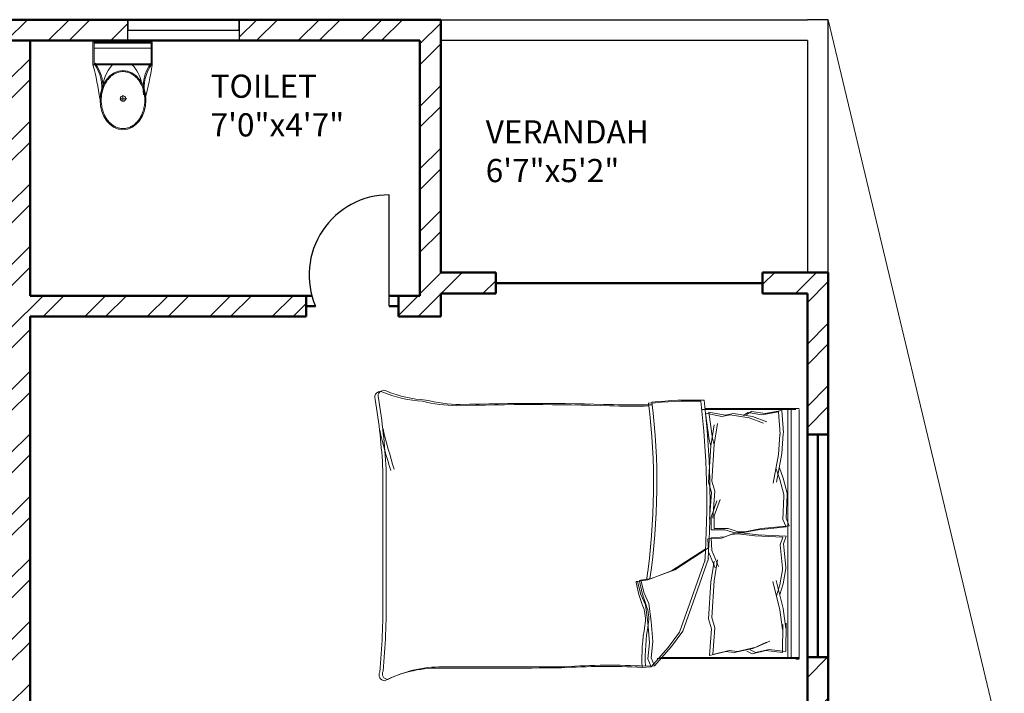
# Model space of a CAD drawing. Units: inches. Extents: x 1901 to 2863, y 888 to 2433.
# Tile 65 of 91: x 2169 to 2381, y 2129 to 2274. Entities that reach past the tile are written whole.
import ezdxf

# ---------------------------------------------------------------- set-up
doc = ezdxf.new("R2010")
doc.units = ezdxf.units.IN
for name, color, linetype, lineweight in [('A-ANNO-SYMB', 8, 'Continuous', 13), ('A-AREA-IDEN', 7, 'Continuous', 18), ('A-DOOR', 4, 'Continuous', 25), ('A-FLOR-FIXT', 9, 'Continuous', 18), ('A-FLOR-HRAL', 41, 'Continuous', 25), ('A-FURN', 8, 'Continuous', 18), ('A-GLAZ', 3, 'Continuous', 25), ('A-WALL', 7, 'Continuous', 50), ('A-WALL-PATT', 8, 'Continuous', 13)]:
    doc.layers.add(name, color=color, linetype=linetype, lineweight=lineweight)
doc.styles.get("Standard").update_dxf_attribs({"font": 'arial.ttf'})

# ---------------------------------------------------------------- blocks, each defined once
blk = doc.blocks.new('A$C31115884')
for p, q in [((257.5, 466.4), (257.5, 523.2)), ((283.1, 497.7), (223.4, 497.7)), ((0, 200), (0, 0)), ((520, 200), (0, 200)), ((10, 190), (10, 10)), ((510, 190), (10, 190)), ((510, 10), (510, 190)), ((520, 0), (520, 200)), ((510, 54.5), (0, 54.5)), ((10, 10), (510, 10)), ((0, 0), (520, 0))]:
    blk.add_line(p, q)
blk.add_circle((255.6, 496.4), 23.6)
for centre, radius, start, end in [((2777.7, -204.6), 2807, 165.4549, 171.71327), ((-294.5, 403.3), 364.7, 324.20913, 9.34987), ((-294.5, 403.3), 374.7, 324.20913, 9.34987), ((805.8, 403.3), 364.7, 170.65013, 215.79087), ((3237, 905), 2807, 188.28673, 194.5451), ((383.6, 406.2), 293.5, 190.27735, 224.15636), ((139.5, 406.2), 293.5, 315.84364, 2.65635), ((805.8, 403.3), 374.7, 179.20365, 215.79087)]:
    blk.add_arc(centre, radius, start, end)
blk.add_ellipse((256.2, 509.9), major_axis=(0, -260.7), ratio=0.772727)
blk.add_open_spline([(256.2, 259.2), (263.1, 259.2), (270, 259.7), (287.8, 262.3), (298.7, 265.1), (319.9, 273.1), (330.2, 278.4), (350.1, 291.1), (359.7, 298.7), (377.7, 315.9), (386.2, 325.5), (401.7, 346.6), (408.8, 358.1), (421.3, 382.5), (426.8, 395.5), (435.9, 422.4), (439.5, 436.4), (444.8, 465.1), (446.5, 479.7), (447.9, 509.2), (447.6, 524), (445, 553.3), (442.7, 567.8), (436.3, 596), (432.1, 609.7), (421.9, 636), (416, 648.6), (402.5, 672.1), (395, 683), (378.6, 703), (369.8, 712.1), (351.1, 728), (341.3, 734.8), (320.9, 746.2), (310.4, 750.7), (288.9, 757.3), (278, 759.4), (256, 761), (245, 760.6), (223.1, 757.2), (212.3, 754.3), (191.1, 746.1), (180.8, 740.7), (160.9, 727.8), (151.4, 720.1), (133.5, 702.7), (125.1, 693), (109.6, 671.7), (102.6, 660.2), (90.2, 635.7), (84.9, 622.7), (76, 595.6), (72.4, 581.6), (67.2, 552.9), (65.6, 538.2), (64.4, 508.8), (64.8, 494), (67.5, 464.7), (69.9, 450.2), (76.6, 422), (80.8, 408.3), (91.1, 382.2), (97.2, 369.7), (110.8, 346.3), (118.4, 335.4), (134.8, 315.6), (143.7, 306.7), (162.4, 290.9), (172.3, 284.2), (192.8, 273), (203.3, 268.6), (224.8, 262.2), (235.8, 260.2), (249.9, 259.3), (253, 259.2), (256.2, 259.2)], degree=3, knots=[0, 0, 0, 0, 0.110105, 0.110105, 0.285049, 0.285049, 0.459994, 0.459994, 0.634938, 0.634938, 0.809882, 0.809882, 0.984827, 0.984827, 1.159771, 1.159771, 1.334715, 1.334715, 1.50966, 1.50966, 1.684604, 1.684604, 1.859549, 1.859549, 2.034493, 2.034493, 2.209437, 2.209437, 2.384382, 2.384382, 2.559326, 2.559326, 2.73427, 2.73427, 2.909215, 2.909215, 3.084159, 3.084159, 3.259103, 3.259103, 3.434048, 3.434048, 3.608992, 3.608992, 3.783936, 3.783936, 3.958881, 3.958881, 4.133825, 4.133825, 4.30877, 4.30877, 4.483714, 4.483714, 4.658658, 4.658658, 4.833603, 4.833603, 5.008547, 5.008547, 5.183491, 5.183491, 5.358436, 5.358436, 5.53338, 5.53338, 5.708324, 5.708324, 5.883269, 5.883269, 6.058213, 6.058213, 6.233158, 6.233158, 6.283185, 6.283185, 6.283185, 6.283185])
blk = doc.blocks.new('BED-DOUBLE')
for p, q in [((31.9, 59.58), (28.25, 55.42)), ((31.9, 59.58), (28.25, 55.42)), ((33.85, 59.67), (31.9, 59.58, 4.35)), ((33.85, 59.67), (31.9, 59.58, 4.35)), ((32.59, 57.85), (31.9, 59.58)), ((32.59, 57.85), (31.9, 59.58)), ((0.03, 57.78), (0.03, 4.12)), ((0.74, 57.78), (30.62, 57.78)), ((0.74, 57.78), (30.62, 57.78)), ((31.18, 59.32), (27.53, 55.16)), ((31.18, 59.32), (27.53, 55.16)), ((33.14, 59.41), (31.18, 59.32, 4.35)), ((33.14, 59.41), (31.18, 59.32, 4.35)), ((31.87, 57.59), (31.18, 59.32)), ((31.87, 57.59), (31.18, 59.32)), ((31.53, 54.12), (31.87, 57.59)), ((31.53, 54.12), (31.87, 57.59)), ((32.24, 54.37), (32.59, 57.85)), ((32.24, 54.37), (32.59, 57.85)), ((2.9, 56.23), (2.79, 50.16)), ((2.9, 56.23), (2.79, 50.16)), ((2.9, 56.23), (6.5, 55.8)), ((2.9, 56.23), (6.5, 55.8)), ((3.61, 56.48), (3.51, 50.42)), ((3.61, 56.48), (3.51, 50.42)), ((3.61, 56.48), (7.22, 56.06)), ((3.61, 56.48), (7.22, 56.06)), ((9.3, 55.33), (6.29, 54)), ((9.3, 55.33), (6.29, 54)), ((6.5, 55.8), (9.39, 56.47)), ((6.5, 55.8), (9.39, 56.47)), ((10.01, 55.58), (7.01, 54.26)), ((10.01, 55.58), (7.01, 54.26)), ((7.22, 56.06), (10.11, 56.73)), ((7.22, 56.06), (10.11, 56.73)), ((13.31, 56.23), (9.3, 55.33)), ((13.31, 56.23), (9.3, 55.33)), ((9.39, 56.47), (10.56, 55.89)), ((9.39, 56.47), (10.56, 55.89)), ((14.02, 56.48), (10.01, 55.58)), ((14.02, 56.48), (10.01, 55.58)), ((10.11, 56.73), (11.28, 56.15)), ((10.11, 56.73), (11.28, 56.15)), ((15.11, 56.01), (13.31, 56.23)), ((15.11, 56.01), (13.31, 56.23)), ((15.83, 56.27), (14.02, 56.48)), ((15.83, 56.27), (14.02, 56.48)), ((18.63, 56.89), (15.11, 56.01)), ((18.63, 56.88), (15.11, 56.01)), ((19.35, 57.14), (15.83, 56.27)), ((19.35, 57.14), (15.83, 56.27)), ((18.18, 51.12), (18.63, 56.89)), ((18.18, 51.12), (18.63, 56.88)), ((18.9, 51.38), (19.35, 57.14)), ((18.9, 51.38), (19.35, 57.14)), ((28.25, 55.42), (25.81, 52.11)), ((28.25, 55.42), (25.81, 52.11)), ((27.53, 55.16), (25.1, 51.86)), ((27.53, 55.16), (25.1, 51.86)), ((31.87, 49.77), (31.53, 54.12)), ((31.87, 49.77), (31.53, 54.12)), ((32.59, 50.03), (32.24, 54.37)), ((32.59, 50.03), (32.24, 54.37)), ((2.79, 50.16), (2.88, 51.29)), ((2.79, 50.16), (2.88, 51.29)), ((2.88, 51.29), (3.47, 47.02)), ((2.88, 51.29), (3.47, 47.02)), ((3.51, 50.42), (3.6, 51.54)), ((3.51, 50.42), (3.6, 51.54)), ((3.6, 51.54), (4.19, 47.28)), ((3.6, 51.54), (4.19, 47.28)), ((18.81, 48.92), (18.18, 51.12)), ((18.81, 48.92), (18.18, 51.12)), ((19.52, 49.18), (18.9, 51.38)), ((19.52, 49.18), (18.9, 51.38)), ((25.1, 51.86), (22.84, 45.6)), ((25.1, 51.86), (22.84, 45.6)), ((25.81, 52.11), (23.55, 45.85)), ((25.81, 52.11), (23.55, 45.85)), ((18.32, 41.05), (18.81, 48.92)), ((18.32, 41.05), (18.81, 48.92)), ((19.04, 41.31), (19.52, 49.18)), ((19.04, 41.31), (19.52, 49.18)), ((32.39, 45.94), (31.87, 49.77)), ((32.39, 45.94), (31.87, 49.77)), ((33.11, 46.2), (32.59, 50.03)), ((33.11, 46.2), (32.59, 50.03)), ((3.47, 47.02), (4.99, 40.94)), ((3.47, 47.02), (4.99, 40.94)), ((4.19, 47.28), (5.71, 41.19)), ((4.19, 47.28), (5.71, 41.19)), ((22.84, 45.6), (19.54, 36.24)), ((22.84, 45.6), (19.54, 36.24)), ((23.55, 45.85), (20.26, 36.49)), ((23.55, 45.85), (20.26, 36.49)), ((33.44, 43.68), (32.39, 45.94)), ((33.44, 43.68), (32.39, 45.94)), ((34.15, 43.94), (33.11, 46.2)), ((34.15, 43.94), (33.11, 46.2)), ((89.72, 17.13), (89.72, 44.77)), ((89.72, 17.13), (89.72, 44.77)), ((4.15, 43.98), (3.48, 41.66)), ((4.15, 43.98), (3.48, 41.66)), ((4.87, 44.23), (4.2, 41.91)), ((4.87, 44.23), (4.2, 41.91)), ((34.13, 40.9), (33.44, 43.68)), ((34.13, 40.9), (33.44, 43.68)), ((34.85, 41.16), (34.15, 43.94)), ((34.85, 41.16), (34.15, 43.94)), ((89, 16.88), (89, 44.51)), ((89, 16.88), (89, 44.51)), ((3.48, 41.66), (2.87, 38.37)), ((3.48, 41.66), (2.87, 38.37)), ((4.2, 41.91), (3.59, 38.62)), ((4.2, 41.91), (3.59, 38.62)), ((17.57, 36.53), (18.32, 41.05)), ((17.57, 36.52), (18.32, 41.05)), ((18.29, 36.78), (19.04, 41.31)), ((18.29, 36.78), (19.04, 41.31)), ((26.83, 38.64), (31.87, 40.55)), ((26.83, 38.64), (31.87, 40.55)), ((27.55, 38.9), (32.59, 40.81)), ((27.55, 38.9), (32.59, 40.81)), ((31.87, 40.55), (34.13, 40.9)), ((31.87, 40.55), (34.13, 40.9)), ((32.59, 40.81), (34.85, 41.16)), ((32.59, 40.81), (34.85, 41.16)), ((2.87, 38.37), (2.9, 38.01)), ((2.87, 38.37), (2.9, 38.01)), ((3.59, 38.62), (3.62, 38.26)), ((3.59, 38.62), (3.62, 38.26)), ((3.62, 38.26), (4.09, 33.29)), ((3.62, 38.26), (4.09, 33.29)), ((19.54, 33.94), (26.83, 38.64)), ((19.54, 33.94), (26.83, 38.64)), ((20.26, 34.19), (27.55, 38.9)), ((20.26, 34.19), (27.55, 38.9)), ((2.9, 38.01), (3.37, 33.03)), ((2.9, 38.01), (3.37, 33.04)), ((18.82, 34.49), (17.38, 37.94)), ((18.82, 34.49), (17.38, 37.94)), ((19.54, 34.74), (18.1, 38.19)), ((19.54, 34.74), (18.1, 38.19)), ((18.99, 31.73), (18.82, 34.49)), ((18.99, 31.73), (18.82, 34.49)), ((19.71, 31.99), (19.54, 34.74)), ((19.71, 31.99), (19.54, 34.74)), ((3.37, 33.04), (2.82, 31.37)), ((3.37, 33.03), (2.82, 31.37)), ((4.09, 33.29), (3.54, 31.63)), ((4.09, 33.29), (3.54, 31.63)), ((16.71, 31.8), (19.71, 31.99)), ((16.71, 31.8), (19.71, 31.99)), ((2.13, 29.14), (8.13, 29.78)), ((2.13, 29.14), (8.13, 29.78)), ((2.82, 31.37), (8.86, 31.1)), ((2.82, 31.37), (8.86, 31.1)), ((2.84, 29.39), (8.85, 30.04)), ((2.84, 29.39), (8.85, 30.04)), ((3.54, 31.63), (9.58, 31.36)), ((3.54, 31.63), (9.58, 31.36)), ((8.13, 29.78), (11.7, 30.43)), ((8.13, 29.78), (11.7, 30.43)), ((8.85, 30.04), (12.42, 30.69)), ((8.85, 30.04), (12.42, 30.69)), ((8.86, 31.1), (12.46, 30.68)), ((8.86, 31.1), (12.46, 30.68)), ((9.58, 31.36), (13.18, 30.93)), ((9.58, 31.36), (13.18, 30.93)), ((11.7, 30.43), (13.16, 30.43)), ((11.7, 30.43), (13.16, 30.43)), ((12.42, 30.69), (13.88, 30.69)), ((12.42, 30.69), (13.88, 30.69)), ((12.46, 30.68), (13.92, 30.77)), ((12.46, 30.68), (13.92, 30.77)), ((13.16, 30.43), (15.28, 29.78)), ((13.16, 30.43), (15.28, 29.78)), ((13.18, 30.93), (14.64, 31.02)), ((13.18, 30.93), (14.64, 31.02)), ((13.88, 30.69), (15.99, 30.04)), ((13.88, 30.69), (15.99, 30.04)), ((13.92, 30.77), (15.99, 31.55)), ((13.92, 30.77), (15.99, 31.55)), ((14.64, 31.02), (16.71, 31.8)), ((14.64, 31.02), (16.71, 31.8)), ((15.28, 29.78), (18.29, 29.78)), ((15.28, 29.78), (18.29, 29.78)), ((15.99, 31.55), (18.99, 31.73)), ((15.99, 31.55), (18.99, 31.73)), ((15.99, 30.04), (19, 30.04)), ((15.99, 30.04), (19, 30.04)), ((18.29, 29.78), (18.29, 27.03)), ((18.29, 29.78), (18.29, 27.03)), ((19, 30.04), (19, 27.28)), ((19, 30.04), (19, 27.28)), ((2.78, 27.51), (2.13, 29.14)), ((2.78, 27.51), (2.13, 29.14)), ((3.49, 27.77), (2.84, 29.39)), ((3.49, 27.77), (2.84, 29.39)), ((3.33, 22.78), (3.49, 27.77)), ((3.33, 22.78), (3.49, 27.77)), ((18.9, 21.98), (19.35, 27.75)), ((18.9, 21.98), (19.35, 27.74)), ((2.61, 22.52), (2.78, 27.51)), ((2.61, 22.52), (2.78, 27.51)), ((18.29, 27.03), (17.06, 23.49)), ((18.29, 27.03), (17.06, 23.5)), ((19, 27.28), (17.78, 23.75)), ((19, 27.28), (17.78, 23.75)), ((18.18, 21.73), (18.63, 27.49)), ((18.18, 21.73), (18.63, 27.49)), ((2.61, 22.16), (2.61, 22.52)), ((2.61, 22.16), (2.61, 22.52)), ((3.42, 18.91), (2.61, 22.16)), ((3.42, 18.91), (2.61, 22.16)), ((3.33, 22.42), (3.33, 22.78)), ((3.33, 22.42), (3.33, 22.78)), ((4.14, 19.17), (3.33, 22.42)), ((4.14, 19.17), (3.33, 22.42)), ((18.81, 19.53), (18.18, 21.73)), ((18.81, 19.53), (18.18, 21.73)), ((19.52, 19.78), (18.9, 21.98)), ((19.52, 19.78), (18.9, 21.98)), ((3.75, 13.56), (4.89, 19.73)), ((3.75, 13.56), (4.89, 19.73)), ((4.95, 16.9), (4.14, 19.17)), ((4.95, 16.9), (4.14, 19.17)), ((4.47, 13.81), (5.6, 19.98)), ((4.47, 13.81), (5.6, 19.98)), ((18.32, 11.66), (18.81, 19.53)), ((18.32, 11.66), (18.81, 19.53)), ((19.04, 11.91), (19.52, 19.78)), ((19.04, 11.91), (19.52, 19.78)), ((4.24, 16.64), (3.42, 18.91)), ((4.24, 16.64), (3.42, 18.91)), ((3.42, 9.27), (3.75, 13.56)), ((3.42, 9.27), (3.75, 13.56)), ((4.14, 9.52), (4.47, 13.81)), ((4.14, 9.52), (4.47, 13.81)), ((17.57, 7.13), (18.32, 11.66)), ((17.57, 7.13), (18.32, 11.66)), ((18.29, 7.38), (19.04, 11.91)), ((18.29, 7.39), (19.04, 11.91)), ((18.32, 11.66), (18.68, 10.38)), ((18.32, 11.66), (18.68, 10.38)), ((19.04, 11.91), (19.4, 10.64)), ((19.04, 11.91), (19.4, 10.64)), ((19.4, 10.64), (20.21, 4.92)), ((19.4, 10.64), (20.21, 4.92)), ((3.4, 9.15), (3.42, 9.27)), ((3.4, 9.15), (3.42, 9.27)), ((3.77, 4.34), (3.4, 9.15)), ((3.77, 4.34), (3.4, 9.15)), ((4.12, 9.4), (4.14, 9.52)), ((4.12, 9.4), (4.14, 9.52)), ((4.49, 4.6), (4.12, 9.4)), ((4.49, 4.6), (4.12, 9.4)), ((18.68, 10.38), (19.5, 4.66)), ((18.68, 10.38), (19.5, 4.66)), ((10.08, 5.63), (7, 6.77)), ((10.08, 5.63), (7, 6.77)), ((10.8, 5.89), (7.71, 7.03)), ((10.8, 5.89), (7.71, 7.03)), ((3.75, 4.34), (7.32, 4.99)), ((3.75, 4.34), (7.32, 4.99)), ((4.47, 4.59), (8.04, 5.24)), ((4.47, 4.59), (8.04, 5.24)), ((7.32, 4.99), (10.24, 4.5)), ((7.32, 4.99), (10.24, 4.5)), ((8.04, 5.24), (10.96, 4.75)), ((8.04, 5.24), (10.96, 4.76)), ((14.14, 4.99), (10.08, 5.63)), ((14.14, 4.99), (10.08, 5.63)), ((10.24, 4.5), (11.38, 5.15)), ((10.24, 4.5), (11.38, 5.15)), ((14.86, 5.24), (10.8, 5.89)), ((14.86, 5.24), (10.8, 5.89)), ((10.96, 4.76), (12.1, 5.4)), ((10.96, 4.75), (12.1, 5.4)), ((15.92, 5.31), (14.14, 4.99)), ((15.92, 5.31), (14.14, 4.99)), ((16.64, 5.57), (14.86, 5.24)), ((16.64, 5.57), (14.86, 5.24)), ((19.5, 4.66), (15.92, 5.31)), ((19.5, 4.66), (15.92, 5.31)), ((20.21, 4.92), (16.64, 5.57)), ((20.21, 4.92), (16.64, 5.57))]:
    blk.add_line(p, q)
for centre, radius, start, end in [((77.12, 85.47), 25.9, 267.4714, 296.4681), ((77.12, 85.47), 25.9, 267.4714, 296.4681), ((77.84, 85.73), 25.9, 267.4714, 296.4681), ((77.84, 85.73), 25.9, 267.4714, 296.4681), ((88.58, 61.05), 1.24, 332.6588, 86.02), ((88.58, 61.05), 1.24, 332.6588, 86.02), ((89.3, 61.31), 1.24, 332.6588, 86.02), ((89.3, 61.31), 1.24, 332.6588, 86.02), ((40.8, 204.6), 145.39, 266.9791, 273.8365), ((40.8, 204.6), 145.39, 266.9791, 273.8365), ((-6.73, 57.85), 40.62, 349.8763, 2.5657), ((-6.73, 57.85), 40.62, 349.8763, 2.5657), ((41.52, 204.86), 145.39, 266.9791, 273.8365), ((41.52, 204.86), 145.39, 266.9791, 273.8365), ((76.17, -5062.23), 5121.82, 90.00217, 90.28689), ((76.17, -5062.23), 5121.82, 90.00217, 90.28689), ((76.89, -5061.97), 5121.82, 90.00217, 90.28689), ((76.89, -5061.97), 5121.82, 90.00217, 90.28689), ((238.36, 46.17), 149.37, 174.4998, 180.6351), ((238.36, 46.17), 149.37, 174.4998, 180.6351), ((239.08, 46.42), 149.37, 174.4998, 180.6351), ((239.08, 46.42), 149.37, 174.4998, 180.6351), ((-7.45, 57.59), 40.62, 349.8763, 2.5657), ((-7.45, 57.59), 40.62, 349.8763, 2.5657), ((39.4, 49.08), 6.99, 168.6608, 203.7384), ((39.4, 49.08), 6.99, 168.6608, 203.7384), ((40.11, 49.33), 6.99, 168.6608, 203.7384), ((40.11, 49.33), 6.99, 168.6608, 203.7384), ((1.69, 34.94), 33.29, 10.6617, 19.8806), ((1.69, 34.94), 33.29, 10.6617, 19.8806), ((2.41, 35.2), 33.29, 10.6617, 19.8806), ((2.41, 35.2), 33.29, 10.6617, 19.8806), ((175.53, 19.9), 144.86, 171.7845, 186.9006), ((175.53, 19.9), 144.86, 171.7845, 186.9006), ((176.25, 20.16), 144.86, 171.7845, 186.9006), ((176.25, 20.15), 144.86, 171.7845, 186.9006), ((34.2, 41.1), 0.207, 250.2464, 1.1377), ((34.2, 41.1), 0.207, 250.2464, 1.1377), ((34.92, 41.35), 0.207, 250.2464, 1.1377), ((34.92, 41.35), 0.207, 250.2464, 1.1377), ((204.43, 23.94), 185.22, 176.0865, 186.7821), ((204.43, 23.94), 185.22, 176.0865, 186.7821), ((205.14, 24.2), 185.22, 176.0865, 186.7821), ((205.14, 24.2), 185.22, 176.0865, 186.7821), ((226.23, 24.28), 136.7, 182.9958, 189.4091), ((226.23, 24.28), 136.7, 182.9958, 189.4091), ((225.52, 24.02), 136.7, 182.9958, 189.4091), ((225.52, 24.02), 136.7, 182.9958, 189.4091), ((22.59, 95.58), 93.53, 268.7218, 275.604), ((22.59, 95.58), 93.53, 268.7218, 275.604), ((23.31, 95.84), 93.53, 268.7218, 275.604), ((23.31, 95.84), 93.53, 268.7218, 275.604), ((35.03, -187.88), 190.99, 88.4762, 91.0082), ((35.03, -187.88), 190.99, 88.4762, 91.0082), ((35.74, -187.62), 190.99, 88.4762, 91.0082), ((35.74, -187.62), 190.99, 88.4762, 91.0082), ((56.85, 544.3), 541.51, 268.2277, 271.7185), ((56.85, 544.3), 541.51, 268.2277, 271.7185), ((57.57, 544.55), 541.51, 268.2277, 271.7185), ((57.57, 544.55), 541.51, 268.2277, 271.7185), ((72.46, -30.24), 33.27, 76.0648, 88.9113), ((72.46, -30.24), 33.27, 76.0648, 88.9113), ((73.18, -29.98), 33.27, 76.0648, 88.9113), ((73.18, -29.98), 33.27, 76.0648, 88.9113), ((79.65, -24.1), 26.45, 67.9751, 86.652), ((79.65, -24.1), 26.45, 67.9751, 86.652), ((78.93, -24.35), 26.45, 67.9751, 86.652), ((78.93, -24.35), 26.45, 67.9751, 86.652), ((89.53, 1.18), 1.22, 236.1736, 23.4781), ((89.53, 1.18), 1.22, 236.1736, 23.4781), ((90.25, 1.44), 1.22, 236.1736, 23.4781), ((90.25, 1.44), 1.22, 236.1736, 23.4781)]:
    blk.add_arc(centre, radius, start, end)
blk = doc.blocks.new('WIN-24-3')
for p, q in [((0, 0), (0, 4.5)), ((0, 4.5), (0, 2.25)), ((24, 2.25), (24, 4.5)), ((24, 4.5), (24, 0)), ((0, 2.25), (24, 2.25))]:
    blk.add_line(p, q)

msp = doc.modelspace()

# ---------------------------------------------------------------- hatches: boundary and pattern name
at = {"layer": 'A-WALL-PATT'}
h = msp.add_hatch(dxfattribs=at)
h.set_pattern_fill('ANSI32', color=256)
h.paths.add_polyline_path([(2192.5, 2274.13), (2141.26, 2274.13), (2141.26, 2269.63), (2192.5, 2269.63)])
h.paths.add_polyline_path([(2259.93, 2274.13), (2216.5, 2274.13), (2216.5, 2269.63), (2255.43, 2269.63), (2255.43, 2214.63), (2250.81, 2214.63), (2250.81, 2210.13), (2259.93, 2210.13), (2259.93, 2215.13), (2271.76, 2215.13), (2271.76, 2217.38), (2271.76, 2219.63), (2259.93, 2219.63)])
h.paths.add_polyline_path([(2171.43, 2269.63), (2166.93, 2269.63), (2166.93, 2219.63), (2121.24, 2219.63), (2121.24, 2215.13), (2166.93, 2215.13), (2166.93, 2083.13), (2161.81, 2083.13), (2161.81, 2078.63), (2171.43, 2078.63), (2177, 2078.63), (2177, 2080.88), (2177, 2083.13), (2171.43, 2083.13), (2171.43, 2210.13), (2230.91, 2210.13), (2230.91, 2212.38), (2230.91, 2214.63), (2171.43, 2214.63)])
h.paths.add_polyline_path([(2117.26, 2274.13), (2089.43, 2274.13), (2089.43, 2219.63), (2081.14, 2219.63), (2081.14, 2215.13), (2089.43, 2215.13), (2098, 2215.13), (2098, 2217.38), (2098, 2219.63), (2093.93, 2219.63), (2093.93, 2269.63), (2117.26, 2269.63), (2117.26, 2271.88)])
h.paths.add_polyline_path([(2343.43, 2219.63), (2329.29, 2219.63), (2329.29, 2215.13), (2338.93, 2215.13), (2338.93, 2184.74), (2343.43, 2184.74)])
h.paths.add_polyline_path([(2338.93, 2083.13), (2329.29, 2083.13), (2208.97, 2083.13), (2208.97, 2078.63), (2338.93, 2078.63)])
h.paths.add_polyline_path([(2343.43, 2136.74), (2338.93, 2136.74), (2338.93, 1872.63), (2343.43, 1872.63)])
h.paths.add_polyline_path([(2343.43, 1863.63), (2397.68, 1863.63), (2397.68, 1821.63), (2384.14, 1821.63), (2384.14, 1812.63), (2418.33, 1812.63), (2418.33, 1817.13), (2418.33, 1821.63), (2406.68, 1821.63), (2406.68, 1863.63), (2459.5, 1863.63), (2459.5, 1821.63), (2447.14, 1821.63), (2447.14, 1812.63), (2459.5, 1812.63), (2468.5, 1812.63), (2468.5, 1872.63), (2394.43, 1872.63), (2334.43, 1872.63), (2334.43, 1812.63), (2343.43, 1812.63), (2353.25, 1812.63), (2353.25, 1821.63), (2343.43, 1821.63)])
h.paths.add_polyline_path([(2510.01, 1872.63), (2468.5, 1872.63), (2468.5, 1868.13), (2510.01, 1868.13)])
h.paths.add_polyline_path([(2514.01, 1817.13), (2468.5, 1817.13), (2468.5, 1812.63), (2482.11, 1812.63), (2482.11, 1800.61), (2486.61, 1800.61), (2486.61, 1812.63), (2514.01, 1812.63)])
h.paths.add_polyline_path([(2299.25, 1814.88), (2299.25, 1817.13), (2295.93, 1817.13), (2295.93, 1854.17), (2293.68, 1854.17), (2291.43, 1854.17), (2291.43, 1817.13), (2266.11, 1817.13), (2266.11, 1812.63), (2299.25, 1812.63)])
h.paths.add_polyline_path([(2218.11, 1817.13), (2206.46, 1817.13), (2171.43, 1817.13), (2171.43, 1949.13), (2190.1, 1949.13), (2190.1, 1953.63), (2163.47, 1953.63), (2163.47, 1949.13), (2166.93, 1949.13), (2166.93, 1817.13), (2114.3, 1817.13), (2114.3, 1812.63), (2218.11, 1812.63)])
h.paths.add_polyline_path([(2029.43, 1970.92), (2024.93, 1970.92), (2024.93, 1912.72), (2029.43, 1912.72)])
h.paths.add_polyline_path([(2132.3, 1953.63), (2113.93, 1953.63), (2113.93, 1975.89), (2111.68, 1975.89), (2109.43, 1975.89), (2109.43, 1953.63), (2029.43, 1953.63), (2029.43, 1949.13), (2132.3, 1949.13)])
h.paths.add_polyline_path([(2029.43, 1853.61), (2029.31, 1853.61), (2029.31, 1853.61), (2029.43, 1853.61), (2029.43, 1864.72), (2024.93, 1864.72), (2024.93, 1812.63), (2066.3, 1812.63), (2066.3, 1814.88), (2066.3, 1817.13), (2029.43, 1817.13)])
h.paths.add_polyline_path([(2122.93, 2010.09), (2120.68, 2010.09), (2118.43, 2010.09), (2118.43, 2006.13), (2029.43, 2006.13), (2029.43, 2001.63), (2109.43, 2001.63), (2109.43, 1998.04), (2113.93, 1998.04), (2113.93, 2001.63), (2122.93, 2001.63)])
h.paths.add_polyline_path([(2029.43, 2031.38), (2024.93, 2031.38), (2024.93, 1994.92), (2027.18, 1994.92), (2029.43, 1994.92)])
h.paths.add_polyline_path([(2029.43, 2136.74), (2024.93, 2136.74), (2024.93, 2067.38), (2027.18, 2067.38), (2029.43, 2067.38)])
h.paths.add_polyline_path([(2125.62, 2083.13), (2029.43, 2083.13), (2029.43, 2078.63), (2118.43, 2078.63), (2118.43, 2030.71), (2122.93, 2030.71), (2122.93, 2078.63), (2125.62, 2078.63)])
h.paths.add_polyline_path([(2029.43, 2215.13), (2040.47, 2215.13), (2040.47, 2217.38), (2040.47, 2219.63), (2024.93, 2219.63), (2024.93, 2184.74), (2029.43, 2184.74), (2029.43, 2187.78)])
h.paths.add_polyline_path([(2686.43, 2274.13), (2659.28, 2274.13), (2659.28, 2269.63), (2681.93, 2269.63), (2681.93, 2219.63), (2676.82, 2219.63), (2676.82, 2215.13), (2681.93, 2215.13), (2697.01, 2215.13), (2697.01, 2217.38), (2697.01, 2219.63), (2686.43, 2219.63)])
h.paths.add_polyline_path([(2609.93, 2269.63), (2635.28, 2269.63), (2635.28, 2274.13), (2571.43, 2274.13), (2571.43, 2269.63), (2605.43, 2269.63), (2605.43, 2214.63), (2549.1, 2214.63), (2549.1, 2210.13), (2605.43, 2210.13), (2605.43, 2083.13), (2601.01, 2083.13), (2601.01, 2080.88), (2601.01, 2078.63), (2609.93, 2078.63), (2616.16, 2078.63), (2616.16, 2080.88), (2616.16, 2083.13), (2609.93, 2083.13), (2609.93, 2215.13), (2651.46, 2215.13), (2651.46, 2217.38), (2651.46, 2219.63), (2609.93, 2219.63)])
h.paths.add_polyline_path([(2521.43, 2269.63), (2547.43, 2269.63), (2547.43, 2271.88), (2547.43, 2274.13), (2516.93, 2274.13), (2516.93, 2219.63), (2506.41, 2219.63), (2506.41, 2215.13), (2516.93, 2215.13), (2516.93, 2210.13), (2525.4, 2210.13), (2525.4, 2212.38), (2525.4, 2214.63), (2521.43, 2214.63)])
h.paths.add_polyline_path([(2456.01, 2219.63), (2439.43, 2219.63), (2439.43, 2187.89), (2443.93, 2187.89), (2443.93, 2215.13), (2456.01, 2215.13)])
h.paths.add_polyline_path([(2752.93, 2219.63), (2739.48, 2219.63), (2739.48, 2215.13), (2748.43, 2215.13), (2748.43, 2187.89), (2752.93, 2187.89)])
h.paths.add_polyline_path([(2752.93, 2139.89), (2748.43, 2139.89), (2748.43, 2083.13), (2648.42, 2083.13), (2648.42, 2078.63), (2654.93, 2078.63), (2654.93, 2039.44), (2659.43, 2039.44), (2659.43, 2078.63), (2748.43, 2078.63), (2748.43, 2063.43), (2752.93, 2063.43)])
h.paths.add_polyline_path([(2752.93, 2010.63), (2659.43, 2010.63), (2659.43, 2015.65), (2654.93, 2015.65), (2654.93, 2010.63), (2605.43, 2010.63), (2605.43, 1920.97), (2609.93, 1920.97), (2609.93, 2006.13), (2748.43, 2006.13), (2748.43, 1982.47), (2752.93, 1982.47)])
h.paths.add_polyline_path([(2752.93, 2027.43), (2748.43, 2027.43), (2748.43, 2010.63), (2752.93, 2010.63)])
h.paths.add_polyline_path([(2748.43, 1886.13), (2609.93, 1886.13), (2609.93, 1889.72), (2605.43, 1889.72), (2605.43, 1861.26), (2609.93, 1861.26), (2609.93, 1881.63), (2748.43, 1881.63)])
h.paths.add_polyline_path([(2456.86, 2228.83), (2498.4, 2228.83), (2498.4, 2247.49), (2456.86, 2247.49)], flags=9)
h.paths.add_polyline_path([(2038.6, 2237.42), (2080.17, 2237.42), (2080.17, 2256.08), (2038.6, 2256.08)], flags=9)
h.paths.add_polyline_path([(2292.01, 1062.39), (2539.93, 1062.39), (2539.93, 1099.49), (2292.01, 1099.49)], flags=9)
h.paths.add_polyline_path([(2424.91, 1832.25), (2448.51, 1832.25), (2448.51, 1846.68), (2424.91, 1846.68)], flags=25)
h.paths.add_polyline_path([(2359.08, 1832.25), (2382.68, 1832.25), (2382.68, 1846.68), (2359.08, 1846.68)], flags=25)
h.paths.add_polyline_path([(2352.9, 1684.8), (2367.54, 1684.8), (2367.54, 1697.17), (2352.9, 1697.17)], flags=9)
h.paths.add_polyline_path([(2079.29, 1755.83), (2169.02, 1755.83), (2169.02, 1774.37), (2079.29, 1774.37)], flags=9)
h.paths.add_polyline_path([(2404.09, 1373.86), (2404.09, 1463.59), (2385.54, 1463.59), (2385.54, 1373.86)], flags=9)
h.paths.add_polyline_path([(2268.09, 2236.37), (2309.64, 2236.37), (2309.64, 2255.03), (2268.09, 2255.03)], flags=9)
h.paths.add_polyline_path([(2575.96, 1700.95), (2665.7, 1700.95), (2665.7, 1719.5), (2575.96, 1719.5)], flags=9)
h.paths.add_polyline_path([(2302.96, 1878.47), (2329.52, 1878.47), (2329.52, 1888.78), (2302.96, 1888.78)], flags=9)
h.paths.add_polyline_path([(2097.42, 2240.58), (2126.57, 2240.58), (2126.57, 2259.23), (2097.42, 2259.23)], flags=9)
h.paths.add_polyline_path([(2208.72, 2246.12), (2237.88, 2246.12), (2237.88, 2264.78), (2208.72, 2264.78)], flags=9)
h.paths.add_polyline_path([(2038.15, 1925.96), (2076.99, 1925.96), (2076.99, 1944.62), (2038.15, 1944.62)], flags=9)
h.paths.add_polyline_path([(2239.14, 1926.67), (2288.46, 1926.67), (2288.46, 1945.33), (2239.14, 1945.33)], flags=9)
h.paths.add_polyline_path([(2175.43, 2007.33), (2212.36, 2007.33), (2212.36, 2025.99), (2175.43, 2025.99)], flags=9)
h.paths.add_polyline_path([(2225.03, 2091.79), (2263.87, 2091.79), (2263.87, 2110.45), (2225.03, 2110.45)], flags=9)
h.paths.add_polyline_path([(2035.4, 2098.48), (2074.24, 2098.48), (2074.24, 2117.14), (2035.4, 2117.14)], flags=9)
h.paths.add_polyline_path([(2050.1, 2029.21), (2083.26, 2029.21), (2083.26, 2047.87), (2050.1, 2047.87)], flags=9)
h.paths.add_polyline_path([(2069.68, 1956.72), (2098.83, 1956.72), (2098.83, 1975.38), (2069.68, 1975.38)], flags=25)
h.paths.add_polyline_path([(2328.62, 1753.34), (2361.66, 1753.34), (2361.66, 1771.99), (2328.62, 1771.99)], flags=9)
h.paths.add_polyline_path([(2395.16, 2060.89), (2395.16, 2140.65), (2378.68, 2140.65), (2378.68, 2060.89)], flags=9)
h.paths.add_polyline_path([(2463.73, 2059.02), (2492.89, 2059.02), (2492.89, 2077.68), (2463.73, 2077.68)], flags=9)
h.paths.add_polyline_path([(2458.03, 2181.54), (2496.87, 2181.54), (2496.87, 2200.19), (2458.03, 2200.19)], flags=9)
h.paths.add_polyline_path([(2527.58, 2243.07), (2556.73, 2243.07), (2556.73, 2261.73), (2527.58, 2261.73)], flags=9)
h.paths.add_polyline_path([(2694.46, 2232.77), (2736.03, 2232.77), (2736.03, 2251.42), (2694.46, 2251.42)], flags=9)
h.paths.add_polyline_path([(2637.82, 2249.22), (2666.98, 2249.22), (2666.98, 2267.88), (2637.82, 2267.88)], flags=9)
h.paths.add_polyline_path([(2623.69, 2183.54), (2662.53, 2183.54), (2662.53, 2202.2), (2623.69, 2202.2)], flags=9)
h.paths.add_polyline_path([(2691.97, 2021.5), (2725.12, 2021.5), (2725.12, 2040.16), (2691.97, 2040.16)], flags=9)
h.paths.add_polyline_path([(2621.04, 1975.91), (2662.34, 1975.91), (2662.34, 1994.57), (2621.04, 1994.57)], flags=25)
h.paths.add_polyline_path([(2479.03, 1927.62), (2519.84, 1927.62), (2519.84, 1946.28), (2479.03, 1946.28)], flags=9)
h.paths.add_polyline_path([(2670.94, 1849.08), (2716.01, 1849.08), (2716.01, 1867.73), (2670.94, 1867.73)], flags=9)
h.paths.add_polyline_path([(2523.61, 1782.96), (2550.17, 1782.96), (2550.17, 1793.26), (2523.61, 1793.26)], flags=9)
h.paths.add_polyline_path([(2450.84, 1207.33), (2492.39, 1207.33), (2492.39, 1225.99), (2450.84, 1225.99)], flags=9)
h.paths.add_polyline_path([(2527.75, 1203.84), (2556.91, 1203.84), (2556.91, 1222.5), (2527.75, 1222.5)], flags=9)
h.paths.add_polyline_path([(2639.11, 1207.2), (2668.27, 1207.2), (2668.27, 1225.86), (2639.11, 1225.86)], flags=9)
h.paths.add_polyline_path([(2692.59, 1218.97), (2734.17, 1218.97), (2734.17, 1237.62), (2692.59, 1237.62)], flags=9)
h.paths.add_polyline_path([(2669.27, 1366.33), (2708.11, 1366.33), (2708.11, 1384.99), (2669.27, 1384.99)], flags=9)
h.paths.add_polyline_path([(2463.31, 1358.03), (2502.15, 1358.03), (2502.15, 1376.69), (2463.31, 1376.69)], flags=9)
h.paths.add_polyline_path([(2494.72, 1449.96), (2531.65, 1449.96), (2531.65, 1468.62), (2494.72, 1468.62)], flags=9)
h.paths.add_polyline_path([(2675.57, 1422.16), (2708.72, 1422.16), (2708.72, 1440.81), (2675.57, 1440.81)], flags=9)
h.paths.add_polyline_path([(2685.63, 1493.89), (2714.79, 1493.89), (2714.79, 1512.55), (2685.63, 1512.55)], flags=9)
h.paths.add_polyline_path([(2686.8, 1529.91), (2725.65, 1529.91), (2725.65, 1548.57), (2686.8, 1548.57)], flags=9)
h.paths.add_polyline_path([(2503.65, 1537.99), (2552.97, 1537.99), (2552.97, 1556.65), (2503.65, 1556.65)], flags=9)
h.paths.add_polyline_path([(2291.71, 1643.5), (2318.28, 1643.5), (2318.28, 1653.81), (2291.71, 1653.81)], flags=9)
h.paths.add_polyline_path([(2450.63, 1610.52), (2477.19, 1610.52), (2477.19, 1620.82), (2450.63, 1620.82)], flags=9)
h.paths.add_polyline_path([(2359.99, 1551.81), (2422.25, 1551.81), (2422.25, 1562.12), (2359.99, 1562.12)], flags=9)
h.paths.add_polyline_path([(2280.11, 1249.01), (2321.65, 1249.01), (2321.65, 1267.66), (2280.11, 1267.66)], flags=9)
h.paths.add_polyline_path([(2164.06, 1274.23), (2193.22, 1274.23), (2193.22, 1292.89), (2164.06, 1292.89)], flags=9)
h.paths.add_polyline_path([(2118.21, 1277.69), (2151.25, 1277.69), (2151.25, 1296.35), (2118.21, 1296.35)], flags=9)
h.paths.add_polyline_path([(2031.95, 1268.53), (2073.52, 1268.53), (2073.52, 1287.19), (2031.95, 1287.19)], flags=9)
h.paths.add_polyline_path([(2050.2, 1409.08), (2089.04, 1409.08), (2089.04, 1427.74), (2050.2, 1427.74)], flags=9)
h.paths.add_polyline_path([(2243.74, 1421.03), (2282.58, 1421.03), (2282.58, 1439.69), (2243.74, 1439.69)], flags=9)
h.paths.add_polyline_path([(2190.75, 1509.77), (2231.56, 1509.77), (2231.56, 1528.43), (2190.75, 1528.43)], flags=9)
h.paths.add_polyline_path([(2058.39, 1475.42), (2091.55, 1475.42), (2091.55, 1494.07), (2058.39, 1494.07)], flags=9)
h.paths.add_polyline_path([(2062.45, 1553.09), (2091.6, 1553.09), (2091.6, 1571.75), (2062.45, 1571.75)], flags=9)
h.paths.add_polyline_path([(2219.52, 1590.37), (2266.15, 1590.37), (2266.15, 1609.02), (2219.52, 1609.02)], flags=9)
h.paths.add_polyline_path([(2041.07, 1584.19), (2079.91, 1584.19), (2079.91, 1602.85), (2041.07, 1602.85)], flags=9)
h = msp.add_hatch(dxfattribs=at)
h.set_pattern_fill('ANSI32', color=256)
h.paths.add_polyline_path([(2443.93, 2139.89), (2439.43, 2139.89), (2439.43, 2069.35), (2441.68, 2069.35), (2443.93, 2069.35), (2443.93, 2078.63), (2521.93, 2078.63), (2521.93, 2075.07), (2524.18, 2075.07), (2526.43, 2075.07), (2526.43, 2078.63), (2571.75, 2078.63), (2571.75, 2080.88), (2571.75, 2083.13), (2443.93, 2083.13)])
h.paths.add_polyline_path([(2526.43, 2054.63), (2524.18, 2054.63), (2521.93, 2054.63), (2521.93, 2030.63), (2443.93, 2030.63), (2443.93, 2045.35), (2439.43, 2045.35), (2439.43, 1983.87), (2443.93, 1983.87), (2443.93, 2026.13), (2521.93, 2026.13), (2526.43, 2026.13)])
h.paths.add_polyline_path([(2443.93, 1923.87), (2439.43, 1923.87), (2439.43, 1872.63), (2443.93, 1872.63)])
h.paths.add_polyline_path([(2636.23, 1766.13), (2609.93, 1766.13), (2609.93, 1779.79), (2605.43, 1779.79), (2605.43, 1766.13), (2486.61, 1766.13), (2486.61, 1770.67), (2482.11, 1770.67), (2482.11, 1766.13), (2482.11, 1761.63), (2636.23, 1761.63), (2636.23, 1763.88)])
h.paths.add_polyline_path([(2519.54, 1663.38), (2519.54, 1665.63), (2494.93, 1665.63), (2481.83, 1665.63), (2481.83, 1663.38), (2481.83, 1661.13), (2490.43, 1661.13), (2490.43, 1640.16), (2494.93, 1640.16), (2494.93, 1661.13), (2519.54, 1661.13)])
h.paths.add_polyline_path([(2443.93, 1712.13), (2443.93, 1716.63), (2414.46, 1716.63), (2414.46, 1712.13), (2439.43, 1712.13), (2439.43, 1545.51), (2443.93, 1545.51), (2443.93, 1661.13), (2448.47, 1661.13), (2448.47, 1665.63), (2443.93, 1665.63)])
h.paths.add_polyline_path([(2343.43, 1712.13), (2365.52, 1712.13), (2365.52, 1714.38), (2365.52, 1716.63), (2333.87, 1716.63), (2333.87, 1714.38), (2333.87, 1712.13), (2338.93, 1712.13), (2338.93, 1575.63), (2338.93, 1545.51), (2343.43, 1545.51), (2343.43, 1547.51), (2343.43, 1580.13)])
h.paths.add_polyline_path([(2752.93, 1665.63), (2579.54, 1665.63), (2579.54, 1661.13), (2615.93, 1661.13), (2615.93, 1529.13), (2598.93, 1529.13), (2598.93, 1524.63), (2623.13, 1524.63), (2623.13, 1526.88), (2623.13, 1529.13), (2620.43, 1529.13), (2620.43, 1661.13), (2748.43, 1661.13), (2748.43, 1633.5), (2752.93, 1633.5)])
h.paths.add_polyline_path([(2752.93, 1419.93), (2748.43, 1419.93), (2748.43, 1400.13), (2659.43, 1400.13), (2659.43, 1444.33), (2657.18, 1444.33), (2654.93, 1444.33), (2654.93, 1400.13), (2643.65, 1400.13), (2643.65, 1395.63), (2748.43, 1395.63), (2748.43, 1364.04), (2752.93, 1364.04)])
h.paths.add_polyline_path([(2752.93, 1492.88), (2748.43, 1492.88), (2748.43, 1476.63), (2667.43, 1476.63), (2667.43, 1479.71), (2665.18, 1479.71), (2662.93, 1479.71), (2662.93, 1476.63), (2654.93, 1476.63), (2654.93, 1469.54), (2659.43, 1469.54), (2659.43, 1472.13), (2748.43, 1472.13), (2748.43, 1455.93), (2752.93, 1455.93)])
h.paths.add_polyline_path([(2752.93, 1304.04), (2748.43, 1304.04), (2748.43, 1263.63), (2738.66, 1263.63), (2738.66, 1259.13), (2752.93, 1259.13)])
h.paths.add_polyline_path([(2685.93, 1259.13), (2695.49, 1259.13), (2695.49, 1261.38), (2695.49, 1263.63), (2677.84, 1263.63), (2677.84, 1261.38), (2677.84, 1259.13), (2681.43, 1259.13), (2681.43, 1203.63), (2653.28, 1203.63), (2653.28, 1199.13), (2685.93, 1199.13), (2685.93, 1203.63)])
h.paths.add_polyline_path([(2609.43, 1395.63), (2611.85, 1395.63), (2611.85, 1400.13), (2598.89, 1400.13), (2598.89, 1397.88), (2598.89, 1395.63), (2604.93, 1395.63), (2604.93, 1268.13), (2554.73, 1268.13), (2554.73, 1265.88), (2554.73, 1263.63), (2604.93, 1263.63), (2604.93, 1203.63), (2571.31, 1203.63), (2571.31, 1199.13), (2604.93, 1199.13), (2629.28, 1199.13), (2629.28, 1201.38), (2629.28, 1203.63), (2609.43, 1203.63), (2609.43, 1258.63), (2609.43, 1259.13), (2654.8, 1259.13), (2654.8, 1263.63), (2609.43, 1263.63)])
h.paths.add_polyline_path([(2443.93, 1304.04), (2439.43, 1304.04), (2439.43, 1259.13), (2443.93, 1259.13), (2456.16, 1259.13), (2456.16, 1261.38), (2456.16, 1263.63), (2443.93, 1263.63)])
h.paths.add_polyline_path([(2525.43, 1263.63), (2531.78, 1263.63), (2531.78, 1268.13), (2520.93, 1268.13), (2520.93, 1263.63), (2511.41, 1263.63), (2511.41, 1259.13), (2520.93, 1259.13), (2520.93, 1199.13), (2547.31, 1199.13), (2547.31, 1201.38), (2547.31, 1203.63), (2525.43, 1203.63)])
h.paths.add_polyline_path([(2443.93, 1434.84), (2439.43, 1434.84), (2439.43, 1364.04), (2441.68, 1364.04), (2443.93, 1364.04)])
h.paths.add_polyline_path([(2567.13, 1400.13), (2443.93, 1400.13), (2443.93, 1395.63), (2567.13, 1395.63)])
h.paths.add_polyline_path([(2443.93, 1545.51), (2439.43, 1545.51), (2439.43, 1494.84), (2443.93, 1494.84)])
h.paths.add_polyline_path([(2494.93, 1553.35), (2492.68, 1553.35), (2490.43, 1553.35), (2490.43, 1524.63), (2494.93, 1524.63), (2525.94, 1524.63), (2525.94, 1526.88), (2525.94, 1529.13), (2494.93, 1529.13)])
h.paths.add_polyline_path([(2752.93, 1573.5), (2748.43, 1573.5), (2748.43, 1529.13), (2657.76, 1529.13), (2657.76, 1524.63), (2662.93, 1524.63), (2662.93, 1498.63), (2667.43, 1498.63), (2667.43, 1524.63), (2748.43, 1524.63), (2748.43, 1516.88), (2752.93, 1516.88)])
h.paths.add_polyline_path([(2038.6, 2237.42), (2080.17, 2237.42), (2080.17, 2256.08), (2038.6, 2256.08)], flags=9)
h.paths.add_polyline_path([(2292.01, 1062.39), (2539.93, 1062.39), (2539.93, 1099.49), (2292.01, 1099.49)], flags=9)
h.paths.add_polyline_path([(2424.91, 1832.25), (2448.51, 1832.25), (2448.51, 1846.68), (2424.91, 1846.68)], flags=9)
h.paths.add_polyline_path([(2359.08, 1832.25), (2382.68, 1832.25), (2382.68, 1846.68), (2359.08, 1846.68)], flags=9)
h.paths.add_polyline_path([(2352.9, 1684.8), (2367.54, 1684.8), (2367.54, 1697.17), (2352.9, 1697.17)], flags=9)
h.paths.add_polyline_path([(2079.29, 1755.83), (2169.02, 1755.83), (2169.02, 1774.37), (2079.29, 1774.37)], flags=9)
h.paths.add_polyline_path([(2404.09, 1373.86), (2404.09, 1463.59), (2385.54, 1463.59), (2385.54, 1373.86)], flags=9)
h.paths.add_polyline_path([(2268.09, 2236.37), (2309.64, 2236.37), (2309.64, 2255.03), (2268.09, 2255.03)], flags=9)
h.paths.add_polyline_path([(2575.96, 1700.95), (2665.7, 1700.95), (2665.7, 1719.5), (2575.96, 1719.5)], flags=9)
h.paths.add_polyline_path([(2302.96, 1878.47), (2329.52, 1878.47), (2329.52, 1888.78), (2302.96, 1888.78)], flags=9)
h.paths.add_polyline_path([(2097.42, 2240.58), (2126.57, 2240.58), (2126.57, 2259.23), (2097.42, 2259.23)], flags=9)
h.paths.add_polyline_path([(2208.72, 2246.12), (2237.88, 2246.12), (2237.88, 2264.78), (2208.72, 2264.78)], flags=9)
h.paths.add_polyline_path([(2038.15, 1925.96), (2076.99, 1925.96), (2076.99, 1944.62), (2038.15, 1944.62)], flags=9)
h.paths.add_polyline_path([(2239.14, 1926.67), (2288.46, 1926.67), (2288.46, 1945.33), (2239.14, 1945.33)], flags=9)
h.paths.add_polyline_path([(2175.43, 2007.33), (2212.36, 2007.33), (2212.36, 2025.99), (2175.43, 2025.99)], flags=9)
h.paths.add_polyline_path([(2225.03, 2091.79), (2263.87, 2091.79), (2263.87, 2110.45), (2225.03, 2110.45)], flags=9)
h.paths.add_polyline_path([(2035.4, 2098.48), (2074.24, 2098.48), (2074.24, 2117.14), (2035.4, 2117.14)], flags=9)
h.paths.add_polyline_path([(2050.1, 2029.21), (2083.26, 2029.21), (2083.26, 2047.87), (2050.1, 2047.87)], flags=9)
h.paths.add_polyline_path([(2069.68, 1956.72), (2098.83, 1956.72), (2098.83, 1975.38), (2069.68, 1975.38)], flags=9)
h.paths.add_polyline_path([(2328.62, 1753.34), (2361.66, 1753.34), (2361.66, 1771.99), (2328.62, 1771.99)], flags=9)
h.paths.add_polyline_path([(2395.16, 2060.89), (2395.16, 2140.65), (2378.68, 2140.65), (2378.68, 2060.89)], flags=9)
h.paths.add_polyline_path([(2463.73, 2059.02), (2492.89, 2059.02), (2492.89, 2077.68), (2463.73, 2077.68)], flags=9)
h.paths.add_polyline_path([(2458.03, 2181.54), (2496.87, 2181.54), (2496.87, 2200.19), (2458.03, 2200.19)], flags=9)
h.paths.add_polyline_path([(2456.86, 2228.83), (2498.4, 2228.83), (2498.4, 2247.49), (2456.86, 2247.49)], flags=9)
h.paths.add_polyline_path([(2527.58, 2243.07), (2556.73, 2243.07), (2556.73, 2261.73), (2527.58, 2261.73)], flags=9)
h.paths.add_polyline_path([(2694.46, 2232.77), (2736.03, 2232.77), (2736.03, 2251.42), (2694.46, 2251.42)], flags=9)
h.paths.add_polyline_path([(2637.82, 2249.22), (2666.98, 2249.22), (2666.98, 2267.88), (2637.82, 2267.88)], flags=9)
h.paths.add_polyline_path([(2623.69, 2183.54), (2662.53, 2183.54), (2662.53, 2202.2), (2623.69, 2202.2)], flags=9)
h.paths.add_polyline_path([(2691.97, 2021.5), (2725.12, 2021.5), (2725.12, 2040.16), (2691.97, 2040.16)], flags=9)
h.paths.add_polyline_path([(2621.04, 1975.91), (2662.34, 1975.91), (2662.34, 1994.57), (2621.04, 1994.57)], flags=9)
h.paths.add_polyline_path([(2479.03, 1927.62), (2519.84, 1927.62), (2519.84, 1946.28), (2479.03, 1946.28)], flags=9)
h.paths.add_polyline_path([(2670.94, 1849.08), (2716.01, 1849.08), (2716.01, 1867.73), (2670.94, 1867.73)], flags=9)
h.paths.add_polyline_path([(2523.61, 1782.96), (2550.17, 1782.96), (2550.17, 1793.26), (2523.61, 1793.26)], flags=9)
h.paths.add_polyline_path([(2450.84, 1207.33), (2492.39, 1207.33), (2492.39, 1225.99), (2450.84, 1225.99)], flags=9)
h.paths.add_polyline_path([(2527.75, 1203.84), (2556.91, 1203.84), (2556.91, 1222.5), (2527.75, 1222.5)], flags=9)
h.paths.add_polyline_path([(2639.11, 1207.2), (2668.27, 1207.2), (2668.27, 1225.86), (2639.11, 1225.86)], flags=9)
h.paths.add_polyline_path([(2692.59, 1218.97), (2734.17, 1218.97), (2734.17, 1237.62), (2692.59, 1237.62)], flags=9)
h.paths.add_polyline_path([(2669.27, 1366.33), (2708.11, 1366.33), (2708.11, 1384.99), (2669.27, 1384.99)], flags=25)
h.paths.add_polyline_path([(2463.31, 1358.03), (2502.15, 1358.03), (2502.15, 1376.69), (2463.31, 1376.69)], flags=9)
h.paths.add_polyline_path([(2494.72, 1449.96), (2531.65, 1449.96), (2531.65, 1468.62), (2494.72, 1468.62)], flags=9)
h.paths.add_polyline_path([(2675.57, 1422.16), (2708.72, 1422.16), (2708.72, 1440.81), (2675.57, 1440.81)], flags=25)
h.paths.add_polyline_path([(2685.63, 1493.89), (2714.79, 1493.89), (2714.79, 1512.55), (2685.63, 1512.55)], flags=9)
h.paths.add_polyline_path([(2686.8, 1529.91), (2725.65, 1529.91), (2725.65, 1548.57), (2686.8, 1548.57)], flags=25)
h.paths.add_polyline_path([(2503.65, 1537.99), (2552.97, 1537.99), (2552.97, 1556.65), (2503.65, 1556.65)], flags=9)
h.paths.add_polyline_path([(2291.71, 1643.5), (2318.28, 1643.5), (2318.28, 1653.81), (2291.71, 1653.81)], flags=9)
h.paths.add_polyline_path([(2450.63, 1610.52), (2477.19, 1610.52), (2477.19, 1620.82), (2450.63, 1620.82)], flags=9)
h.paths.add_polyline_path([(2359.99, 1551.81), (2422.25, 1551.81), (2422.25, 1562.12), (2359.99, 1562.12)], flags=9)
h.paths.add_polyline_path([(2280.11, 1249.01), (2321.65, 1249.01), (2321.65, 1267.66), (2280.11, 1267.66)], flags=9)
h.paths.add_polyline_path([(2164.06, 1274.23), (2193.22, 1274.23), (2193.22, 1292.89), (2164.06, 1292.89)], flags=9)
h.paths.add_polyline_path([(2118.21, 1277.69), (2151.25, 1277.69), (2151.25, 1296.35), (2118.21, 1296.35)], flags=9)
h.paths.add_polyline_path([(2031.95, 1268.53), (2073.52, 1268.53), (2073.52, 1287.19), (2031.95, 1287.19)], flags=9)
h.paths.add_polyline_path([(2050.2, 1409.08), (2089.04, 1409.08), (2089.04, 1427.74), (2050.2, 1427.74)], flags=9)
h.paths.add_polyline_path([(2243.74, 1421.03), (2282.58, 1421.03), (2282.58, 1439.69), (2243.74, 1439.69)], flags=9)
h.paths.add_polyline_path([(2190.75, 1509.77), (2231.56, 1509.77), (2231.56, 1528.43), (2190.75, 1528.43)], flags=9)
h.paths.add_polyline_path([(2058.39, 1475.42), (2091.55, 1475.42), (2091.55, 1494.07), (2058.39, 1494.07)], flags=9)
h.paths.add_polyline_path([(2062.45, 1553.09), (2091.6, 1553.09), (2091.6, 1571.75), (2062.45, 1571.75)], flags=9)
h.paths.add_polyline_path([(2219.52, 1590.37), (2266.15, 1590.37), (2266.15, 1609.02), (2219.52, 1609.02)], flags=9)
h.paths.add_polyline_path([(2041.07, 1584.19), (2079.91, 1584.19), (2079.91, 1602.85), (2041.07, 1602.85)], flags=9)

# ---------------------------------------------------------------- linework, layer by layer
at = {"layer": 'A-ANNO-SYMB'}
msp.add_line((2343.43, 2274.13), (2439.43, 1872.63), dxfattribs=at)
at = {"layer": 'A-DOOR'}
msp.add_line((2248.81, 2212.38), (2248.81, 2236.38), dxfattribs=at)
msp.add_arc((2248.81, 2219.12), 17.26, 90, 202.9606, dxfattribs=at)
at = {"layer": 'A-FLOR-HRAL'}
for p, q in [((2259.93, 2274.13), (2338.93, 2274.13)), ((2343.43, 2274.13), (2338.93, 2274.13)), ((2343.43, 2269.63), (2343.43, 2274.13)), ((2338.93, 2269.63), (2259.93, 2269.63)), ((2338.93, 2269.63), (2338.93, 2219.63)), ((2343.43, 2219.63), (2343.43, 2269.63))]:
    msp.add_line(p, q, dxfattribs=at)
at = {"layer": 'A-FURN'}
for p, q in [((2316.08, 2190.09), (2336.42, 2190.09)), ((2316.08, 2190.09), (2336.42, 2190.09)), ((2316.8, 2190.34), (2337.13, 2190.34)), ((2316.8, 2190.34), (2337.13, 2190.34)), ((2334.69, 2190.09), (2334.69, 2136.43)), ((2334.69, 2190.09), (2334.69, 2136.43)), ((2335.41, 2190.34), (2335.41, 2136.69)), ((2335.41, 2190.34), (2335.41, 2136.69)), ((2337.13, 2136.69), (2307.26, 2136.69)), ((2337.13, 2136.69), (2307.26, 2136.69))]:
    msp.add_line(p, q, dxfattribs=at)
for centre in [(2363.04, 2213.32), (2363.04, 2213.32), (2363.76, 2213.58), (2363.76, 2213.58)]:
    msp.add_arc(centre, 119.53, 193.3832, 197.7053, dxfattribs=at)
at = {"layer": 'A-WALL'}
for p, q in [((2089.43, 2274.13), (2259.93, 2274.13)), ((2259.93, 2274.13), (2259.93, 2219.63)), ((2093.93, 2269.63), (2255.43, 2269.63)), ((2171.43, 2269.63), (2171.43, 2214.63)), ((2255.43, 2269.63), (2255.43, 2214.63)), ((2259.93, 2219.63), (2271.76, 2219.63)), ((2271.76, 2219.63), (2271.76, 2215.13)), ((2329.29, 2217.38), (2329.29, 2219.63)), ((2329.29, 2219.63), (2329.29, 2215.13)), ((2329.29, 2219.63), (2343.43, 2219.63)), ((2343.43, 2219.63), (2343.43, 1872.63)), ((2271.76, 2215.13), (2271.76, 2217.38)), ((2271.76, 2217.38), (2329.29, 2217.38)), ((2171.43, 2214.63), (2232.14, 2214.63)), ((2230.91, 2214.63), (2230.91, 2210.13)), ((2248.81, 2214.63), (2255.43, 2214.63)), ((2250.81, 2214.63), (2250.81, 2210.13)), ((2259.93, 2215.13), (2271.76, 2215.13)), ((2259.93, 2215.13), (2259.93, 2210.13)), ((2329.29, 2215.13), (2338.93, 2215.13)), ((2338.93, 2215.13), (2338.93, 1872.63)), ((2230.91, 2210.13), (2230.91, 2212.38)), ((2230.91, 2212.38), (2232.91, 2212.38)), ((2250.81, 2212.38), (2248.81, 2212.38)), ((2250.81, 2210.13), (2250.81, 2212.38)), ((2171.43, 2210.13), (2230.91, 2210.13)), ((2171.43, 2210.13), (2171.43, 2083.13)), ((2250.81, 2210.13), (2259.93, 2210.13)), ((2338.93, 2184.74), (2343.43, 2184.74)), ((2343.43, 2184.74), (2341.18, 2184.74)), ((2341.18, 2184.74), (2341.18, 2136.74)), ((2343.43, 2184.74), (2343.43, 2184.74)), ((2337.13, 2136.43), (2336.42, 2136.43)), ((2341.18, 2136.74), (2338.93, 2136.74)), ((2338.93, 2136.74), (2343.43, 2136.74))]:
    msp.add_line(p, q, dxfattribs=at)

# ---------------------------------------------------------------- block references
at = {"layer": 'A-FLOR-FIXT', "xscale": 0.0245149588751191, "yscale": 0.0245149588751191, "zscale": 0.0245149588751191, "rotation": 180}
msp.add_blockref('A$C31115884', (2197.72, 2269.31), dxfattribs=at)
at = {"layer": 'A-FURN', "rotation": 180}
msp.add_blockref('BED-DOUBLE', (2337.16, 2194.21), dxfattribs=at)
at = {"layer": 'A-GLAZ'}
msp.add_blockref('WIN-24-3', (2192.5, 2269.63), dxfattribs=at)

# ---------------------------------------------------------------- texts
at = {"layer": 'A-AREA-IDEN', "char_height": 5, "attachment_point": 1}
for s, width, insert in [('TOILET\\P7\'0"x4\'7"', 104.0752, (2210.31, 2262.3)), ('VERANDAH\\P6\'7"x5\'2"', 115.0961, (2269.6, 2252.45))]:
    msp.add_mtext_dynamic_manual_height_columns(s, width=width, gutter_width=12.5, heights=[0], dxfattribs=dict(at, insert=insert))

doc.saveas('drawing.dxf')
